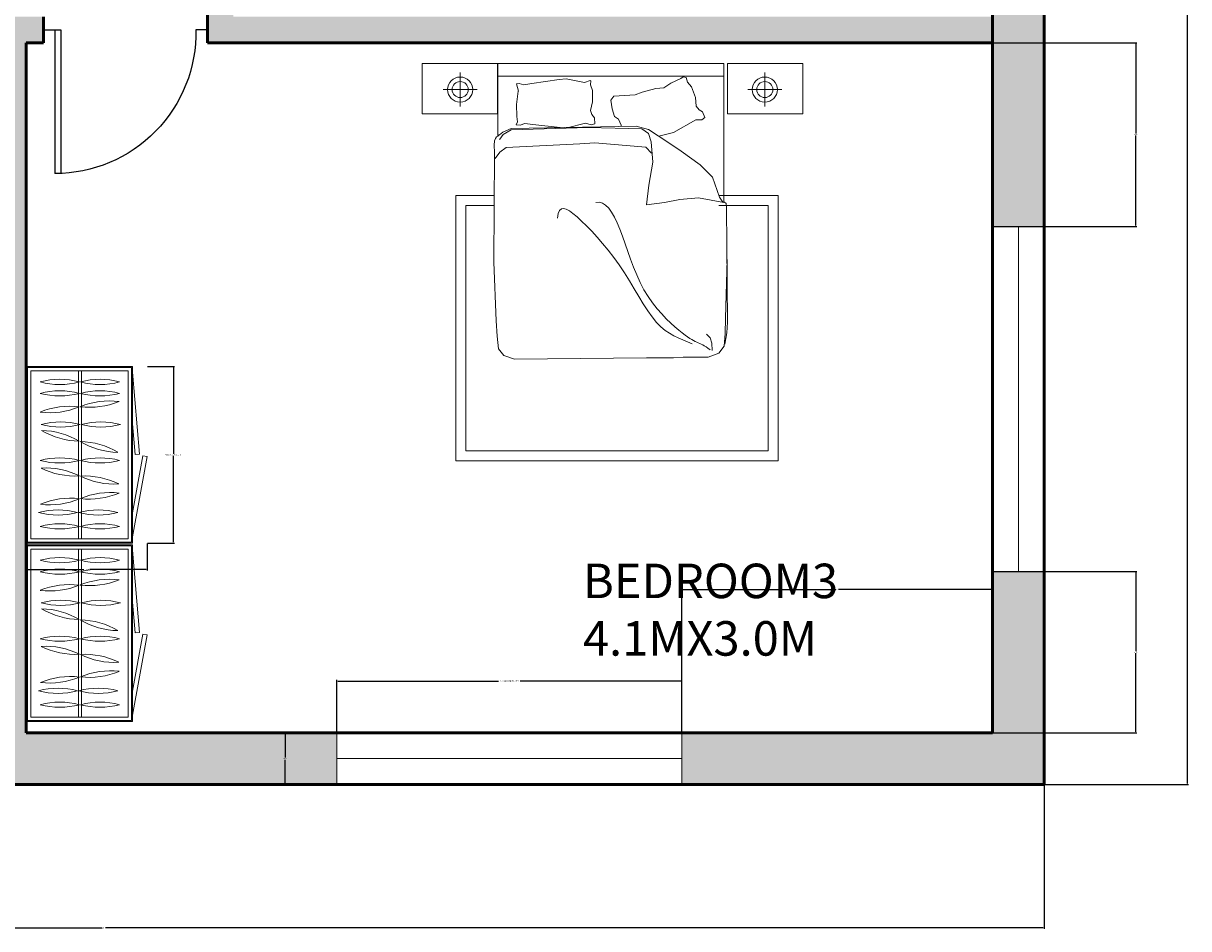
# Model space of a CAD drawing. Units: inches. Extents: x 3 to 380, y -485 to 60.
# Tile 5 of 8: x 177 to 380, y -485 to -328. Entities that reach past the tile are written whole.
import ezdxf

# ---------------------------------------------------------------- set-up
doc = ezdxf.new("R2010")
doc.units = ezdxf.units.IN
doc.header["$MEASUREMENT"] = 0
for name, color, linetype, lineweight in [('A-ANNO-DIMS', 2, 'Continuous', 18), ('A-AREA-IDEN', 7, 'Continuous', 25), ('A-DOOR', 3, 'Continuous', 25), ('A-FURN', 8, 'Continuous', 18), ('A-GLAZ', 4, 'Continuous', 18), ('A-WALL', 7, 'Continuous', 50), ('A-WALL-PATT', 252, 'Continuous', 13)]:
    doc.layers.add(name, color=color, linetype=linetype, lineweight=lineweight)
doc.styles.get("Standard").update_dxf_attribs({"font": 'arial.ttf'})
doc.dimstyles.get("Standard").update_dxf_attribs({"dimtxt": 0.18, "dimasz": 0.18, "dimexe": 0.18, "dimexo": 0.0625, "dimgap": 0.09, "dimtad": 0, "dimtih": 1, "dimtoh": 1, "dimdec": 0, "dimzin": 0, "dimdsep": 46, "dimlunit": 3, "dimtxsty": 'Standard', "dimcen": 0.09, "dimadec": 0, "dimazin": 0, "dimtfac": 1, "dimtdec": 0, "dimtofl": 0, "dimtmove": 0, "dimatfit": 3, "dimfxl": 1, "dimtolj": 1, "dimtzin": 0, "dimarcsym": 0})

# ---------------------------------------------------------------- blocks, each defined once
blk = doc.blocks.new('BED-DOUBLE-WITH-NIGHTSTANDS')
for p, q in [((13.15, 56.48), (13.15, 69.11)), ((6.62, 67.56), (6.62, 61.62)), ((59.58, 67.56), (59.58, 61.62)), ((16.76, 64.3), (16.42, 65.57)), ((25.02, 66.47), (23.83, 66.33)), ((28.24, 65.8), (25.02, 66.47)), ((29.23, 66.16), (28.24, 65.8)), ((29.33, 66.13), (29.23, 66.16)), ((29.33, 66.13), (29.25, 65.4)), ((29.33, 66.13), (29.25, 65.4)), ((29.25, 65.4), (29.65, 64.45)), ((40.63, 64.79), (42.02, 64.91)), ((42.02, 64.91), (43.24, 65.73)), ((42.02, 64.91), (43.24, 65.73)), ((43.24, 65.73), (44.98, 66.53)), ((46.15, 65.85), (46.84, 65.09)), ((46.84, 65.09), (47.51, 63.2)), ((3.65, 64.59), (9.59, 64.59)), ((29.65, 64.45), (29.63, 62.44)), ((33.33, 63.47), (37.02, 63.69)), ((37.02, 63.69), (38.27, 64.16)), ((38.27, 64.16), (40.63, 64.79)), ((47.51, 63.2), (47.67, 61.68)), ((62.55, 64.59), (56.61, 64.59)), ((29.63, 62.44), (29.27, 60.96)), ((29.27, 60.96), (29.52, 60.24)), ((47.67, 61.68), (48.15, 61.09)), ((48.15, 61.09), (48.75, 60.71)), ((29.52, 60.24), (29.96, 59.68)), ((29.96, 59.68), (30.03, 58.63)), ((47.6, 59.3), (43.73, 57.13)), ((48.66, 59.34), (47.6, 59.3)), ((49.17, 59.74), (48.66, 59.34)), ((48.75, 60.71), (49.17, 59.74)), ((28.4, 58.75), (25.21, 57.93)), ((29.41, 58.43), (28.4, 58.75)), ((30.03, 58.63), (29.41, 58.43)), ((12.59, 55.61), (12.54, 55)), ((12.54, 55), (12.56, 53.58)), ((12.56, 53.58), (12.48, 34.55)), ((52.39, 45), (52.46, 45.03)), ((52.97, 37.68), (52.91, 43.85)), ((53.11, 24.16), (52.97, 37.68)), ((12.48, 34.55), (12.89, 24.35)), ((53.02, 35.03), (52.75, 24.82)), ((12.89, 24.35), (13.03, 21.68)), ((52.75, 24.82), (52.69, 22.14)), ((52.63, 20.34), (53, 22.29)), ((53, 22.29), (53.11, 24.16)), ((13.03, 21.68), (13.27, 19.48)), ((50.1, 21.39), (49.46, 22.06)), ((50.39, 20.5), (50.1, 21.39)), ((50.45, 19.2), (50.39, 20.5)), ((52.69, 22.14), (52.52, 19.94)), ((13.27, 19.48), (14.23, 18.32)), ((14.23, 18.32), (16.09, 17.69)), ((51.59, 18.75), (49.75, 18.06)), ((52.52, 19.94), (51.59, 18.75)), ((39.03, 17.94), (16.09, 17.69)), ((39.03, 17.94), (43.71, 17.94)), ((43.71, 17.94), (45.37, 18.06)), ((45.37, 18.06), (49.75, 18.06))]:
    blk.add_line(p, q)
for points in [[(0, 60.38), (13.1, 60.38), (13.1, 69.11), (0, 69.11)], [(66.2, 60.38), (53.1, 60.38), (53.1, 69.11), (66.2, 69.11)]]:
    blk.add_lwpolyline(points, close=True)
for points in [[(13.15, 69.11), (52.45, 69.11), (52.45, 45.06)], [(52.45, 66.93), (13.15, 66.93)], [(23.83, 66.33), (19.08, 65.62), (17.7, 65.39), (16.88, 65.65), (16.42, 65.57)], [(46.15, 65.85), (45.9, 66.66), (45.38, 66.82), (44.98, 66.53)], [(24.02, 58.01), (19.24, 58.51), (17.85, 58.68), (17.04, 58.38), (16.37, 58.47), (16.56, 59), (16.45, 59.9), (16.42, 62), (16.71, 64.3)], [(33.33, 63.47), (32.82, 62.74), (33.06, 61.23), (33.43, 59.89), (34.16, 59.47), (34.58, 58.37), (34.59, 58.17)], [(52.45, 44.97), (48.05, 45.75), (44.8, 45.5), (42.14, 44.97), (38.99, 44.52), (39.41, 47.96), (40.12, 51.96), (39.81, 55.5), (39.35, 56.93), (38.2, 57.74), (28.88, 58), (15.49, 57.6), (14.12, 56.79), (13.54, 55.99), (13.47, 55.91)], [(13.48, 56.71), (14.02, 57.18), (15.49, 57.8), (37.2, 58.22), (39.38, 57.66), (42.87, 55.35), (45.06, 53.9), (48.36, 51.48), (50.46, 49.34), (51.7, 45.9), (52.31, 45)], [(43.73, 57.13), (41.15, 56.49)], [(12.61, 55.65), (12.74, 56.06), (12.92, 56.37), (13.15, 56.48), (13.4, 56.7), (13.44, 56.72)], [(39.86, 53.54), (38.87, 54.55), (30.01, 55.3), (27.42, 55.15), (14.59, 54.51), (13.51, 53.69), (12.69, 52.6)], [(51.61, 46.15), (61.88, 46.15), (61.88, 0), (5.85, 0), (5.85, 46.15), (12.53, 46.15)], [(50.06, 19.34), (49.7, 19.62), (49.37, 19.84), (49.06, 20.03), (48.78, 20.19), (48.52, 20.33), (48.27, 20.44), (48.02, 20.55), (47.76, 20.67), (47.5, 20.79), (47.21, 20.93), (46.9, 21.1), (46.56, 21.31), (46.16, 21.57), (45.71, 21.89), (45.2, 22.29), (44.61, 22.76), (43.95, 23.32), (43.23, 23.98), (42.45, 24.72), (41.66, 25.56), (40.85, 26.48), (40.05, 27.49), (39.29, 28.58), (38.57, 29.76), (37.91, 31.03), (37.31, 32.35), (36.75, 33.71), (36.24, 35.08), (35.75, 36.45), (35.28, 37.79), (34.82, 39.08), (34.36, 40.29), (33.9, 41.4), (33.43, 42.39), (32.94, 43.25), (32.44, 43.96), (31.91, 44.5), (31.37, 44.86), (30.8, 45.01), (30.2, 44.94)], [(52.91, 43.91), (52.84, 44.76), (52.6, 45.01), (52.45, 45.06)], [(51.61, 44.4), (60.14, 44.4), (60.14, 1.75), (7.59, 1.75), (7.59, 44.4), (12.53, 44.4)], [(46.96, 20.37), (46.12, 20.73), (45.31, 21.07), (44.52, 21.41), (43.75, 21.77), (42.99, 22.2), (42.24, 22.71), (41.49, 23.33), (40.74, 24.1), (39.99, 25.04), (39.23, 26.12), (38.46, 27.32), (37.67, 28.61), (36.87, 29.96), (36.03, 31.34), (35.16, 32.73), (34.26, 34.09), (33.32, 35.4), (32.36, 36.66), (31.39, 37.84), (30.42, 38.95), (29.48, 39.98), (28.57, 40.91), (27.72, 41.73), (26.93, 42.45), (26.23, 43.05), (25.61, 43.51), (25.06, 43.81), (24.6, 43.93), (24.22, 43.85), (23.91, 43.56), (23.68, 43.04), (23.52, 42.25)]]:
    blk.add_lwpolyline(points)
for centre, radius in [((6.62, 64.59), 2.18), ((6.62, 64.59), 1.4), ((59.58, 64.59), 2.18), ((59.58, 64.59), 1.4)]:
    blk.add_circle(centre, radius)
blk = doc.blocks.new('WARDROBE-WIDE-MODULE')
for p, q in [((9.04, 29.96), (9.04, 0.74)), ((9.57, 29.96), (9.57, 0.74))]:
    blk.add_line(p, q)
for points in [[(0, 30.7), (0, 0), (18.42, 0), (18.42, 30.7)], [(0.17, 30.53), (0.17, 0.17), (18.25, 0.17), (18.25, 30.53)], [(0.74, 29.96), (0.74, 0.74), (17.68, 0.74), (17.68, 29.96)]]:
    blk.add_lwpolyline(points, close=True)
for points in [[(18.42, 29.74), (19.61, 15.44), (18.86, 15.37), (18.42, 20.73)], [(18.42, 1.09), (20.96, 15.05), (20.23, 15.18), (18.42, 5.25)]]:
    blk.add_lwpolyline(points)
for centre, start, end in [((5.78, 15.16), 75.1905, 104.8095), ((12.78, 15.16), 75.1905, 104.8095), ((5.78, 40.88), 255.1905, 284.8095), ((5.78, 13.16), 75.1905, 104.8095), ((12.78, 40.88), 255.1905, 284.8095), ((12.78, 13.16), 75.1905, 104.8095), ((5.78, 38.89), 255.1905, 284.8095), ((14.4, 11.41), 82.7904, 112.4093), ((11, 36.91), 262.7904, 292.4093), ((12.78, 38.89), 255.1905, 284.8095), ((7.46, 10.48), 82.7904, 112.4093), ((4.06, 35.98), 262.7904, 292.4093), ((5.93, 7.75), 75.1905, 104.8095), ((5.93, 33.48), 255.1905, 284.8095), ((12.92, 7.75), 75.1905, 104.8095), ((12.92, 33.48), 255.1905, 284.8095), ((2.35, 6.27), 59.2346, 88.8535), ((9.43, 31.01), 239.2346, 268.8535), ((16.15, 29.08), 239.2346, 268.8535), ((9.08, 4.34), 59.2346, 88.8535), ((5.78, 1.5), 75.1905, 104.8095), ((5.78, 27.23), 255.1905, 284.8095), ((12.78, 1.5), 75.1905, 104.8095), ((12.78, 27.23), 255.1905, 284.8095), ((3.28, -0.25), 63.6481, 93.267), ((8.42, 24.96), 243.6481, 273.267), ((10.13, -1.65), 63.6481, 93.267), ((15.28, 23.56), 243.6481, 273.267), ((14.57, -4.52), 83.3262, 112.9452), ((10.92, 20.95), 263.3262, 292.9452), ((7.64, -5.51), 83.3262, 112.9452), ((4, 19.96), 263.3262, 292.9452), ((5.47, -7.55), 75.1905, 104.8095), ((5.47, 18.18), 255.1905, 284.8095), ((12.47, -7.55), 75.1905, 104.8095), ((12.47, 18.18), 255.1905, 284.8095), ((5.78, -9.97), 75.1905, 104.8095), ((5.78, 15.76), 255.1905, 284.8095), ((12.78, -9.97), 75.1905, 104.8095), ((12.78, 15.76), 255.1905, 284.8095)]:
    blk.add_arc(centre, 13.31, start, end)
blk = doc.blocks.new('WIN-60X9')
for p, q in [((60, 9), (0, 9)), ((0, 9), (0, 0)), ((60, 0), (60, 9)), ((0, 4.5), (60, 4.5)), ((0, 0), (60, 0))]:
    blk.add_line(p, q)
blk = doc.blocks.new('WIN-60X9-SPLIT-JAMB')
for p, q in [((60, 9), (0, 9)), ((0, 9), (0, 0)), ((60, 4.5), (60, 9)), ((0, 4.5), (60, 4.5)), ((60, 4.5), (60, 0)), ((0, 0), (60, 0))]:
    blk.add_line(p, q)
blk = doc.blocks.new('DOOR-SWING-25')
for p, q in [((2, 0), (2, 25)), ((3, 0), (3, 25)), ((0, 0), (2, 0)), ((2, 0), (3, 0)), ((28.5, 0), (26.5, 0))]:
    blk.add_line(p, q)
blk.add_arc((2, 0.5), 24.5, 358.8425, 90)
blk = doc.blocks.new('*D19')
at = {"layer": 'A-ANNO-DIMS', "color": 0, "lineweight": -2, "transparency": 16777216}
for p, q in [((231.84, -451.27), (231.84, -442.16)), ((232.02, -442.34), (259.96, -442.34)), ((291.66, -442.34), (263.72, -442.34)), ((291.84, -451.27), (291.84, -442.16))]:
    blk.add_line(p, q, dxfattribs=at)
at = {"layer": 'A-ANNO-DIMS', "color": 0, "transparency": 16777216}
for points in [[(232.02, -442.31), (232.02, -442.37), (231.84, -442.34)], [(291.66, -442.31), (291.66, -442.37), (291.84, -442.34)]]:
    blk.add_solid(points, dxfattribs=at)
at = {"layer": 'Defpoints', "color": 0, "transparency": 16777216}
for p in [(291.84, -442.34), (231.84, -451.34), (291.84, -451.34)]:
    blk.add_point(p, dxfattribs=at)
at = {"layer": 'A-ANNO-DIMS', "color": 0, "transparency": 16777216, "insert": (261.84, -442.34), "char_height": 0.18, "attachment_point": 5}
blk.add_mtext('\\A1;SPLIT-JAMB WINDOW 60 TYP.', dxfattribs=at)
blk = doc.blocks.new('*D20')
at = {"layer": 'A-ANNO-DIMS', "color": 0, "lineweight": -2, "transparency": 16777216}
for p, q in [((231.78, -451.34), (222.66, -451.34)), ((222.84, -451.52), (222.84, -455.65)), ((222.84, -460.16), (222.84, -456.02)), ((231.78, -460.34), (222.66, -460.34))]:
    blk.add_line(p, q, dxfattribs=at)
at = {"layer": 'A-ANNO-DIMS', "color": 0, "transparency": 16777216}
for points in [[(222.81, -451.52), (222.87, -451.52), (222.84, -451.34)], [(222.81, -460.16), (222.87, -460.16), (222.84, -460.34)]]:
    blk.add_solid(points, dxfattribs=at)
at = {"layer": 'Defpoints', "color": 0, "transparency": 16777216}
for p in [(222.84, -451.34), (231.84, -451.34), (231.84, -460.34)]:
    blk.add_point(p, dxfattribs=at)
at = {"layer": 'A-ANNO-DIMS', "color": 0, "transparency": 16777216, "insert": (222.84, -455.84), "char_height": 0.18, "attachment_point": 5}
blk.add_mtext('\\A1;9 TYP.', dxfattribs=at)
blk = doc.blocks.new('*D31')
at = {"layer": 'A-ANNO-DIMS', "color": 0, "lineweight": -2, "transparency": 16777216}
for p, q in [((198.93, -387.64), (203.65, -387.64)), ((203.47, -387.82), (203.47, -402.81)), ((203.47, -418.17), (203.47, -403.18)), ((198.93, -418.35), (203.65, -418.35))]:
    blk.add_line(p, q, dxfattribs=at)
at = {"layer": 'A-ANNO-DIMS', "color": 0, "transparency": 16777216}
for points in [[(203.44, -387.82), (203.5, -387.82), (203.47, -387.64)], [(203.44, -418.17), (203.5, -418.17), (203.47, -418.35)]]:
    blk.add_solid(points, dxfattribs=at)
at = {"layer": 'Defpoints', "color": 0, "transparency": 16777216}
for p in [(198.87, -387.64), (203.47, -387.64), (198.87, -418.35)]:
    blk.add_point(p, dxfattribs=at)
at = {"layer": 'A-ANNO-DIMS', "color": 0, "transparency": 16777216, "insert": (203.47, -402.99), "char_height": 0.18, "attachment_point": 5}
blk.add_mtext('\\A1;WIDE WARDROBE 31 TYP.', dxfattribs=at)
blk = doc.blocks.new('*D32')
at = {"layer": 'A-ANNO-DIMS', "color": 0, "lineweight": -2, "transparency": 16777216}
for p, q in [((177.9, -418.41), (177.9, -423.13)), ((198.87, -418.41), (198.87, -423.13)), ((178.08, -422.95), (187.86, -422.95)), ((198.69, -422.95), (188.91, -422.95))]:
    blk.add_line(p, q, dxfattribs=at)
at = {"layer": 'A-ANNO-DIMS', "color": 0, "transparency": 16777216}
for points in [[(178.08, -422.92), (178.08, -422.98), (177.9, -422.95)], [(198.69, -422.92), (198.69, -422.98), (198.87, -422.95)]]:
    blk.add_solid(points, dxfattribs=at)
at = {"layer": 'Defpoints', "color": 0, "transparency": 16777216}
for p in [(177.9, -418.35), (198.87, -418.35), (198.87, -422.95)]:
    blk.add_point(p, dxfattribs=at)
at = {"layer": 'A-ANNO-DIMS', "color": 0, "transparency": 16777216, "insert": (188.39, -422.95), "char_height": 0.18, "attachment_point": 5}
blk.add_mtext('\\A1;21 TYP.', dxfattribs=at)
blk = doc.blocks.new('*D49')
at = {"layer": 'A-ANNO-DIMS', "color": 0, "lineweight": -2, "transparency": 16777216}
for p, q in [((27.84, -460.4), (27.84, -485.42)), ((354.84, -460.4), (354.84, -485.42)), ((28.02, -485.24), (191.05, -485.24)), ((354.66, -485.24), (191.63, -485.24))]:
    blk.add_line(p, q, dxfattribs=at)
at = {"layer": 'A-ANNO-DIMS', "color": 0, "transparency": 16777216}
for points in [[(28.02, -485.21), (28.02, -485.27), (27.84, -485.24)], [(354.66, -485.21), (354.66, -485.27), (354.84, -485.24)]]:
    blk.add_solid(points, dxfattribs=at)
at = {"layer": 'Defpoints', "color": 0, "transparency": 16777216}
for p in [(27.84, -460.34), (354.84, -460.34), (354.84, -485.24)]:
    blk.add_point(p, dxfattribs=at)
at = {"layer": 'A-ANNO-DIMS', "color": 0, "transparency": 16777216, "insert": (191.34, -485.24), "char_height": 0.18, "attachment_point": 5}
blk.add_mtext('\\A1;327', dxfattribs=at)
blk = doc.blocks.new('*D51')
at = {"layer": 'A-ANNO-DIMS', "color": 0, "lineweight": -2, "transparency": 16777216}
for p, q in [((151.9, 34.66), (379.92, 34.66)), ((379.74, 34.48), (379.74, -212.65)), ((379.74, -460.16), (379.74, -213.02)), ((354.9, -460.34), (379.92, -460.34))]:
    blk.add_line(p, q, dxfattribs=at)
at = {"layer": 'A-ANNO-DIMS', "color": 0, "transparency": 16777216}
for points in [[(379.71, 34.48), (379.77, 34.48), (379.74, 34.66)], [(379.71, -460.16), (379.77, -460.16), (379.74, -460.34)]]:
    blk.add_solid(points, dxfattribs=at)
at = {"layer": 'Defpoints', "color": 0, "transparency": 16777216}
for p in [(151.84, 34.66), (354.84, -460.34), (379.74, -460.34)]:
    blk.add_point(p, dxfattribs=at)
at = {"layer": 'A-ANNO-DIMS', "color": 0, "transparency": 16777216, "insert": (379.74, -212.84), "char_height": 0.18, "attachment_point": 5}
blk.add_mtext('\\A1;495', dxfattribs=at)
blk = doc.blocks.new('*D68')
at = {"layer": 'A-ANNO-DIMS', "color": 0, "lineweight": -2, "transparency": 16777216}
for p, q in [((345.9, -331.34), (370.92, -331.34)), ((370.74, -331.52), (370.74, -347.13)), ((370.74, -363.1), (370.74, -347.49)), ((345.9, -363.28), (370.92, -363.28))]:
    blk.add_line(p, q, dxfattribs=at)
at = {"layer": 'A-ANNO-DIMS', "color": 0, "transparency": 16777216}
for points in [[(370.71, -331.52), (370.77, -331.52), (370.74, -331.34)], [(370.71, -363.1), (370.77, -363.1), (370.74, -363.28)]]:
    blk.add_solid(points, dxfattribs=at)
at = {"layer": 'Defpoints', "color": 0, "transparency": 16777216}
for p in [(345.84, -331.34), (345.84, -363.28), (370.74, -363.28)]:
    blk.add_point(p, dxfattribs=at)
at = {"layer": 'A-ANNO-DIMS', "color": 0, "transparency": 16777216, "insert": (370.74, -347.31), "char_height": 0.18, "attachment_point": 5}
blk.add_mtext('\\A1;31.95', dxfattribs=at)
blk = doc.blocks.new('*D69')
at = {"layer": 'A-ANNO-DIMS', "color": 0, "lineweight": -2, "transparency": 16777216}
for p, q in [((345.9, -423.28), (370.92, -423.28)), ((370.74, -423.46), (370.74, -437.13)), ((370.74, -451.16), (370.74, -437.49)), ((345.9, -451.34), (370.92, -451.34))]:
    blk.add_line(p, q, dxfattribs=at)
at = {"layer": 'A-ANNO-DIMS', "color": 0, "transparency": 16777216}
for points in [[(370.71, -423.46), (370.77, -423.46), (370.74, -423.28)], [(370.71, -451.16), (370.77, -451.16), (370.74, -451.34)]]:
    blk.add_solid(points, dxfattribs=at)
at = {"layer": 'Defpoints', "color": 0, "transparency": 16777216}
for p in [(345.84, -423.28), (345.84, -451.34), (370.74, -451.34)]:
    blk.add_point(p, dxfattribs=at)
at = {"layer": 'A-ANNO-DIMS', "color": 0, "transparency": 16777216, "insert": (370.74, -437.31), "char_height": 0.18, "attachment_point": 5}
blk.add_mtext('\\A1;28.05', dxfattribs=at)
blk = doc.blocks.new('*D80')
at = {"layer": 'A-ANNO-DIMS', "color": 0, "lineweight": -2, "transparency": 16777216}
for p, q in [((291.84, -451.27), (291.84, -426.26)), ((292.02, -426.44), (318.62, -426.44)), ((345.66, -426.44), (319.06, -426.44)), ((345.84, -451.27), (345.84, -426.26))]:
    blk.add_line(p, q, dxfattribs=at)
at = {"layer": 'A-ANNO-DIMS', "color": 0, "transparency": 16777216}
for points in [[(292.02, -426.41), (292.02, -426.47), (291.84, -426.44)], [(345.66, -426.41), (345.66, -426.47), (345.84, -426.44)]]:
    blk.add_solid(points, dxfattribs=at)
at = {"layer": 'Defpoints', "color": 0, "transparency": 16777216}
for p in [(345.84, -426.44), (291.84, -451.34), (345.84, -451.34)]:
    blk.add_point(p, dxfattribs=at)
at = {"layer": 'A-ANNO-DIMS', "color": 0, "transparency": 16777216, "insert": (318.84, -426.44), "char_height": 0.18, "attachment_point": 5}
blk.add_mtext('\\A1;54', dxfattribs=at)

msp = doc.modelspace()

# ---------------------------------------------------------------- hatches: boundary and pattern name
at = {"layer": 'A-WALL-PATT'}
h = msp.add_hatch(color=256, dxfattribs=at)
h.dxf.hatch_style = 1
h.paths.add_polyline_path([(36.8404, 6.1643), (51.3404, 6.1643), (51.3404, 15.1643), (27.8404, 15.1643), (27.8404, -143.6318), (36.8404, -143.6318)])
h.paths.add_polyline_path([(125.8404, 10.6643), (125.8404, 15.1643), (111.3404, 15.1643), (111.3404, 6.1643), (125.8404, 6.1643)])
h.paths.add_polyline_path([(170.6358, 15.1643), (153.8404, 15.1643), (153.8404, 6.1643), (156.8404, 6.1643), (156.8404, -82.3357), (173.3404, -82.3357), (173.3404, -130.3357), (177.8404, -130.3357), (180.8404, -130.3357), (180.8404, -125.8357), (177.8404, -125.8357), (177.8404, -82.3357), (201.8404, -82.3357), (201.8404, -38.0857), (197.3404, -38.0857), (197.3404, -77.8357), (161.3404, -77.8357), (161.3404, 6.1643), (170.6358, 6.1643)])
h.paths.add_polyline_path([(241.3739, 15.1643), (194.6358, 15.1643), (194.6358, 6.1643), (241.3739, 6.1643)])
h.paths.add_polyline_path([(201.8404, 6.1643), (197.3404, 6.1643), (197.3404, -12.1977), (201.8404, -12.1977)], flags=17)
h.paths.add_polyline_path([(354.8404, 15.1643), (301.3739, 15.1643), (301.3739, 6.1643), (345.8404, 6.1643), (345.8404, -34.0336), (354.8404, -34.0336)])
h.paths.add_polyline_path([(354.8404, -94.0336), (345.8404, -94.0336), (345.8404, -159.3738), (354.8404, -159.3738)])
h.paths.add_polyline_path([(345.8404, -125.8357), (209.3404, -125.8357), (209.3404, -205.8357), (211.5904, -205.8357), (213.8404, -205.8357), (213.8404, -130.3357), (345.8404, -130.3357)])
h.paths.add_polyline_path([(36.8404, -203.6318), (27.8404, -203.6318), (27.8404, -270.1269), (36.8404, -270.1269)])
h.paths.add_polyline_path([(36.8404, -330.1269), (27.8404, -330.1269), (27.8404, -362.428), (57.3404, -362.428), (57.3404, -353.428), (36.8404, -353.428)])
h.paths.add_polyline_path([(177.8404, -331.3357), (180.8404, -331.3357), (180.8404, -326.8357), (173.3404, -326.8357), (173.3404, -353.428), (165.8404, -353.428), (165.8404, -362.428), (168.8404, -362.428), (168.8404, -451.3357), (168.8404, -460.3357), (231.8404, -460.3357), (231.8404, -451.3357), (177.8404, -451.3357)])
h.paths.add_polyline_path([(354.8404, -305.1003), (345.8404, -305.1003), (345.8404, -363.2829), (354.8404, -363.2829)])
h.paths.add_polyline_path([(345.8404, -326.8357), (213.8404, -326.8357), (213.8404, -312.8357), (211.5904, -312.8357), (209.3404, -312.8357), (209.3404, -331.3357), (345.8404, -331.3357)])
h.paths.add_polyline_path([(345.8404, -262.3357), (237.8404, -262.3357), (237.8404, -233.8357), (209.3404, -233.8357), (209.3404, -284.8357), (213.8404, -284.8357), (213.8404, -238.3357), (233.3404, -238.3357), (233.3404, -266.8357), (345.8404, -266.8357)])
h.paths.add_polyline_path([(354.8404, -219.3738), (345.8404, -219.3738), (345.8404, -281.1003), (354.8404, -281.1003)])
h = msp.add_hatch(color=256, dxfattribs=at)
h.dxf.hatch_style = 1
h.paths.add_polyline_path([(354.8404, -423.2829), (345.8404, -423.2829), (345.8404, -451.3357), (291.8404, -451.3357), (291.8404, -455.8357), (291.8404, -460.3357), (354.8404, -460.3357)])

# ---------------------------------------------------------------- linework, layer by layer
at = {"layer": 'A-WALL'}
for p, q in [((354.8404, 15.1643), (354.8404, -460.3357)), ((345.8404, 6.1643), (345.8404, -451.3357)), ((209.3404, -312.8357), (209.3404, -331.3357)), ((180.8404, -326.8357), (180.8404, -331.3357)), ((177.8404, -331.3357), (177.8404, -451.3357)), ((180.8404, -331.3357), (177.8404, -331.3357)), ((209.3404, -331.3357), (345.8404, -331.3357)), ((177.8404, -451.3357), (345.8404, -451.3357)), ((27.8404, -460.3357), (354.8404, -460.3357))]:
    msp.add_line(p, q, dxfattribs=at)

# ---------------------------------------------------------------- block references
at = {"layer": 'A-DOOR', "extrusion": (0, 0, -1), "zscale": -1, "rotation": 180}
msp.add_blockref('DOOR-SWING-25', (-180.84, -329.0854), dxfattribs=at)
at = {"layer": 'A-FURN'}
for name, p in [('BED-DOUBLE-WITH-NIGHTSTANDS', (246.6711, -404.0748)), ('WARDROBE-WIDE-MODULE', (177.905, -418.3459)), ('WARDROBE-WIDE-MODULE', (177.905, -449.354))]:
    msp.add_blockref(name, p, dxfattribs=at)
at = {"layer": 'A-GLAZ', "rotation": 270.0000000000001}
msp.add_blockref('WIN-60X9', (345.84, -363.283), dxfattribs=at)
at = {"layer": 'A-GLAZ'}
msp.add_blockref('WIN-60X9-SPLIT-JAMB', (231.84, -460.336), dxfattribs=at)

# ---------------------------------------------------------------- texts
at = {"layer": 'A-AREA-IDEN', "insert": (274.628, -421.9312), "char_height": 6, "attachment_point": 1}
msp.add_mtext('BEDROOM3\\P4.1MX3.0M', dxfattribs=at)

# ---------------------------------------------------------------- dimensions: what is measured, and where the dimension line sits
at = {"layer": 'A-ANNO-DIMS'}
for base, p1, p2, angle, override, picture, middle in [((379.7404, -460.3357), (151.8404, 34.6643), (354.8404, -460.3357), 90, {"dimdec": 0, "dimlfac": 1, "dimrnd": 0, "dimzin": 0, "dimdsep": 46, "dimlunit": 2}, '*D51', (379.7404, -212.8357)), ((370.7404, -363.2829), (345.8404, -331.3357), (345.8404, -363.2829), 270, {"dimdec": 2, "dimlfac": 1, "dimrnd": 0, "dimzin": 0, "dimdsep": 46, "dimlunit": 2}, '*D68', (370.7404, -347.3093)), ((370.7404, -451.3357), (345.8404, -423.2829), (345.8404, -451.3357), 270, {"dimdec": 2, "dimlfac": 1, "dimrnd": 0, "dimzin": 0, "dimdsep": 46, "dimlunit": 2}, '*D69', (370.7404, -437.3093))]:
    dim = msp.add_linear_dim(base=base, p1=p1, p2=p2, angle=angle, dimstyle='Standard', override=override, dxfattribs=at)
    dim.commit()
    dim.dimension.update_dxf_attribs({"geometry": picture, "text_midpoint": middle})
for base, p1, p2, text, picture, middle in [((203.471, -387.6434), (198.8656, -418.3464), (198.8656, -387.6434), 'WIDE WARDROBE <> TYP.', '*D31', (203.471, -402.9949)), ((222.8404, -451.3357), (231.8404, -460.3357), (231.8404, -451.3357), '<> TYP.', '*D20', (222.8404, -455.8357))]:
    dim = msp.add_linear_dim(base=base, p1=p1, p2=p2, angle=90, text=text, dimstyle='Standard', override={"dimdec": 0, "dimlfac": 1, "dimrnd": 0, "dimzin": 0, "dimdsep": 46, "dimlunit": 2}, dxfattribs=at)
    dim.commit()
    dim.dimension.update_dxf_attribs({"geometry": picture, "text_midpoint": middle})
for base, p1, p2, text, picture, middle in [((198.8656, -422.9518), (177.9046, -418.3464), (198.8656, -418.3464), '<> TYP.', '*D32', (188.3851, -422.9518)), ((291.8404, -442.3357), (231.8404, -451.3357), (291.8404, -451.3357), 'SPLIT-JAMB WINDOW <> TYP.', '*D19', (261.8404, -442.3357))]:
    dim = msp.add_linear_dim(base=base, p1=p1, p2=p2, text=text, dimstyle='Standard', override={"dimdec": 0, "dimlfac": 1, "dimrnd": 0, "dimzin": 0, "dimdsep": 46, "dimlunit": 2}, dxfattribs=at)
    dim.commit()
    dim.dimension.update_dxf_attribs({"geometry": picture, "text_midpoint": middle})
for base, p1, p2, picture, middle in [((345.8404, -426.4357), (291.8404, -451.3357), (345.8404, -451.3357), '*D80', (318.8404, -426.4357)), ((354.8404, -485.2357), (27.8404, -460.3357), (354.8404, -460.3357), '*D49', (191.3404, -485.2357))]:
    dim = msp.add_linear_dim(base=base, p1=p1, p2=p2, dimstyle='Standard', override={"dimdec": 0, "dimlfac": 1, "dimrnd": 0, "dimzin": 0, "dimdsep": 46, "dimlunit": 2}, dxfattribs=at)
    dim.commit()
    dim.dimension.update_dxf_attribs({"geometry": picture, "text_midpoint": middle})

doc.saveas('drawing.dxf')
